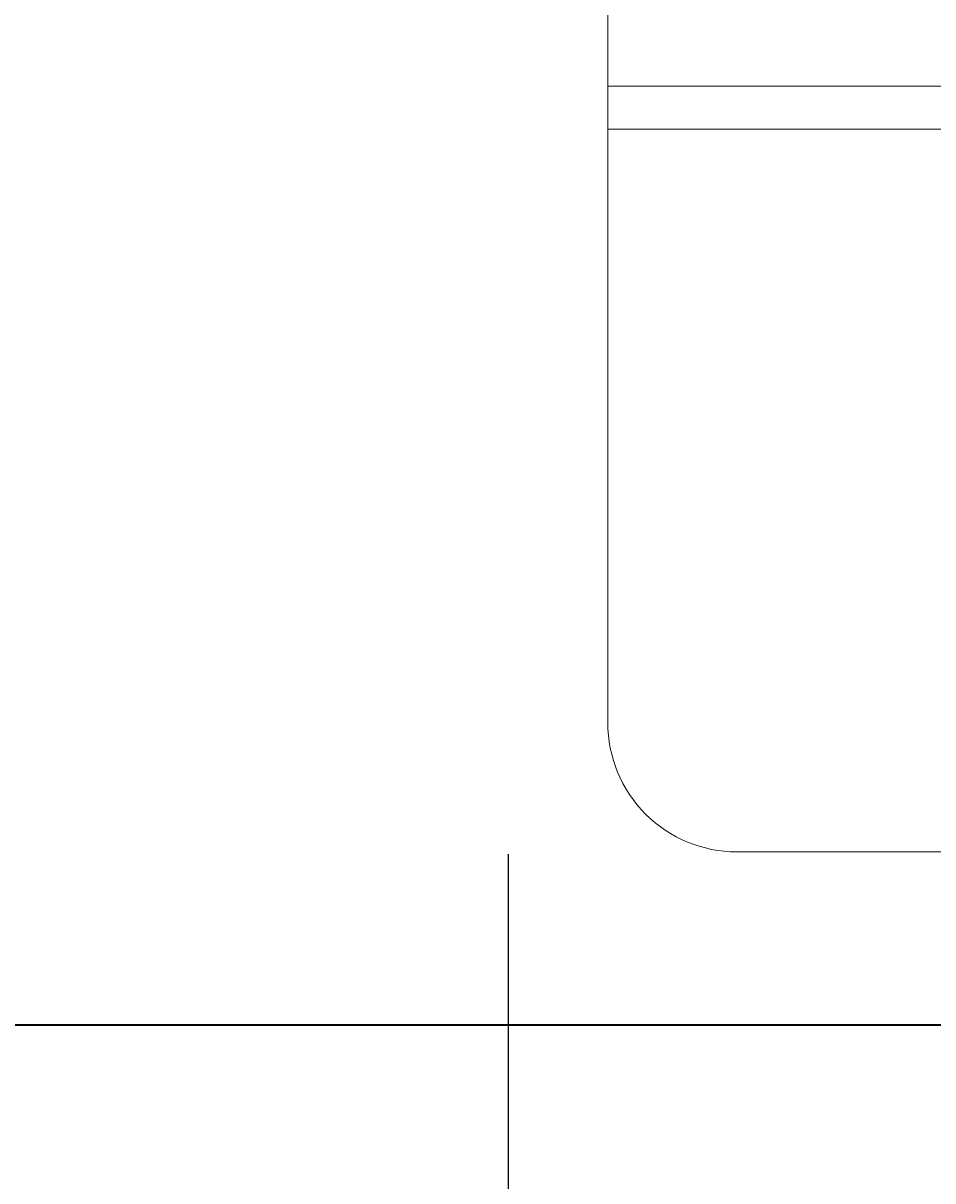
# Model space of a CAD drawing. Units: inches. Extents: x -61 to 1599, y -1316 to 257.
# Tile 4 of 204: x 99 to 123, y -1211 to -1180. Entities that reach past the tile are written whole.
import ezdxf

# ---------------------------------------------------------------- set-up
doc = ezdxf.new("R2010")
doc.units = ezdxf.units.IN
doc.header["$MEASUREMENT"] = 0
for name, color, linetype, lineweight in [('A-ANNO-DIMS', 2, 'Continuous', 18), ('FURNITURE', 83, 'Continuous', 18), ('WALLS', 4, 'Continuous', 35)]:
    doc.layers.add(name, color=color, linetype=linetype, lineweight=lineweight)
doc.styles.get("Standard").update_dxf_attribs({"font": 'arial.ttf'})
doc.dimstyles.get("Standard").update_dxf_attribs({"dimtxt": 0.18, "dimasz": 0.18, "dimexe": 0.18, "dimexo": 0.0625, "dimgap": 0.09, "dimtad": 0, "dimtih": 1, "dimtoh": 1, "dimdec": 0, "dimzin": 0, "dimdsep": 46, "dimlunit": 3, "dimtxsty": 'Standard', "dimcen": 0.09, "dimadec": 0, "dimazin": 0, "dimtfac": 1, "dimtdec": 0, "dimtofl": 0, "dimtmove": 0, "dimatfit": 3, "dimfxl": 1, "dimtolj": 1, "dimtzin": 0, "dimarcsym": 0})

# ---------------------------------------------------------------- blocks, each defined once
blk = doc.blocks.new('BED-DOUBLE')
for p, q in [((1.272, 20.467), (70.263, 20.467)), ((1.272, 19.317), (70.263, 19.317))]:
    blk.add_line(p, q)
blk.add_lwpolyline([(1.272, 88.537), (1.272, 3.449, 0.414214), (4.722, 0), (66.813, 0, 0.414214), (70.263, 3.449), (70.263, 88.537, 0.414214), (66.813, 91.987), (4.722, 91.987, 0.414214)], format="xyb", close=True)
blk = doc.blocks.new('*D635')
at = {"layer": 'A-ANNO-DIMS', "color": 0, "lineweight": -2, "transparency": 16777216}
for p, q in [((111.872, -1202.381), (111.872, -1216.391)), ((183.57, -1202.381), (183.57, -1216.391)), ((112.052, -1216.211), (147.193, -1216.211)), ((183.39, -1216.211), (148.248, -1216.211))]:
    blk.add_line(p, q, dxfattribs=at)
at = {"layer": 'A-ANNO-DIMS', "color": 0, "transparency": 16777216}
for points in [[(112.052, -1216.181), (112.052, -1216.241), (111.872, -1216.211)], [(183.39, -1216.181), (183.39, -1216.241), (183.57, -1216.211)]]:
    blk.add_solid(points, dxfattribs=at)
at = {"layer": 'DEFPOINTS', "color": 0, "transparency": 16777216}
for p in [(111.872, -1202.318), (183.57, -1202.318), (183.57, -1216.211)]:
    blk.add_point(p, dxfattribs=at)
at = {"layer": 'A-ANNO-DIMS', "color": 0, "transparency": 16777216, "insert": (147.721, -1216.211), "char_height": 0.18, "attachment_point": 5}
blk.add_mtext('\\A1;72 TYP.', dxfattribs=at)
blk = doc.blocks.new('*D687')
at = {"layer": 'A-ANNO-DIMS', "color": 0, "lineweight": -2, "transparency": 16777216}
for p, q in [((289.418, 181.677), (-61.077, 181.677)), ((-60.897, 181.497), (-60.897, -528.952)), ((-60.897, -1239.765), (-60.897, -529.316)), ((319.64, -1239.945), (-61.077, -1239.945))]:
    blk.add_line(p, q, dxfattribs=at)
at = {"layer": 'A-ANNO-DIMS', "color": 0, "transparency": 16777216}
for points in [[(-60.927, 181.497), (-60.867, 181.497), (-60.897, 181.677)], [(-60.927, -1239.765), (-60.867, -1239.765), (-60.897, -1239.945)]]:
    blk.add_solid(points, dxfattribs=at)
at = {"layer": 'DEFPOINTS', "color": 0, "transparency": 16777216}
for p in [(289.481, 181.677), (-60.897, -1239.945), (319.703, -1239.945)]:
    blk.add_point(p, dxfattribs=at)
at = {"layer": 'A-ANNO-DIMS', "color": 0, "transparency": 16777216, "insert": (-60.897, -529.134), "char_height": 0.18, "attachment_point": 5}
blk.add_mtext('\\A1;1421.6', dxfattribs=at)

msp = doc.modelspace()

# ---------------------------------------------------------------- linework, layer by layer
at = {"layer": 'WALLS'}
msp.add_line((14.7028, -1206.9446), (237.7028, -1206.9446), dxfattribs=at)

# ---------------------------------------------------------------- block references
at = {"layer": 'FURNITURE'}
msp.add_blockref('BED-DOUBLE', (113.2612, -1202.3177), dxfattribs=at)

# ---------------------------------------------------------------- dimensions: what is measured, and where the dimension line sits
at = {"layer": 'A-ANNO-DIMS'}
dim = msp.add_linear_dim(base=(-60.8972, -1239.9446), p1=(289.4807, 181.6771), p2=(319.7028, -1239.9446), angle=90, dimstyle='Standard', override={"dimdec": 1, "dimlfac": 1, "dimrnd": 0, "dimzin": 0, "dimdsep": 46, "dimlunit": 2}, dxfattribs=at)
dim.commit()
dim.dimension.update_dxf_attribs({"geometry": '*D687', "text_midpoint": (-60.8972, -529.1337)})
dim = msp.add_linear_dim(base=(183.5695, -1216.2111), p1=(111.8719, -1202.3182), p2=(183.5695, -1202.3182), text='<> TYP.', dimstyle='Standard', override={"dimdec": 0, "dimlfac": 1, "dimrnd": 0, "dimzin": 0, "dimdsep": 46, "dimlunit": 2}, dxfattribs=at)
dim.commit()
dim.dimension.update_dxf_attribs({"geometry": '*D635', "text_midpoint": (147.7207, -1216.2111)})

doc.saveas('drawing.dxf')
